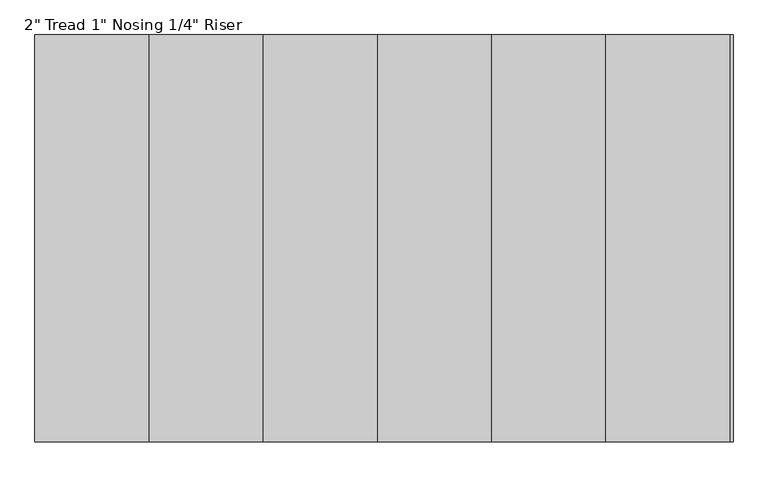
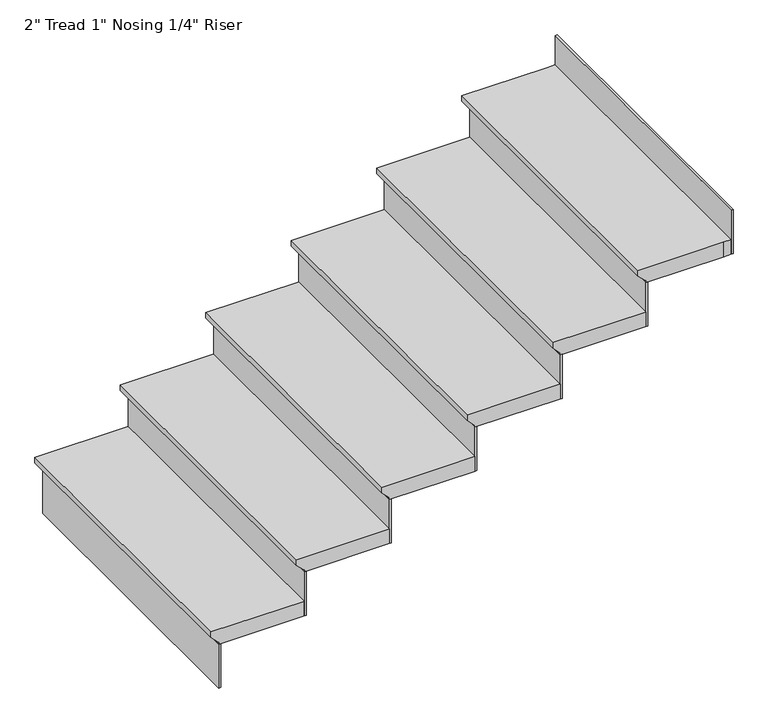
"""IFC4 building model written with IfcOpenShell, lengths in millimetres: stair flight geometry."""

from ifc_helpers import new_model, si_unit, origin, place, context, project, spatial, faceted_brep, source, transform, mapped, element, save


def stair_flight_d80cec9a(model_context):
    return source(origin(), model_context, "Body", "Brep", [
        faceted_brep([(-6729.7502524, 11195.5128362, 1352.55), (-6729.7502524, 11195.5128362, 1371.6), (-6729.7502524, 12192.4628362, 1371.6), (-6729.7502524, 12192.4628362, 1352.55), (-6704.3502524, 11195.5128362, 1327.15), (-6704.3502524, 12192.4628362, 1327.15), (-6424.9502524, 11195.5128362, 1371.6), (-6424.9502524, 12192.4628362, 1371.6), (-6704.3502524, 12192.4628362, 1320.8), (-6424.9502524, 12192.4628362, 1320.8), (-6424.9502524, 11195.5128362, 1320.8), (-6704.3502524, 11195.5128362, 1320.8)], [[[0, 1, 2, 3]], [[4, 0, 3, 5]], [[2, 1, 6, 7]], [[8, 9, 10, 11]], [[2, 7, 9, 8, 5, 3]], [[8, 11, 4, 5]], [[6, 1, 0, 4, 11, 10]], [[7, 6, 10, 9]]]),
        faceted_brep([(-6704.3502524, 11195.5128362, 1320.8), (-6704.3502524, 11195.5128362, 1168.4), (-6698.0002524, 11195.5128362, 1168.4), (-6698.0002524, 11195.5128362, 1320.8), (-6704.3502524, 12192.4628362, 1320.8), (-6698.0002524, 12192.4628362, 1320.8), (-6698.0002524, 12192.4628362, 1168.4), (-6704.3502524, 12192.4628362, 1168.4)], [[[0, 1, 2, 3]], [[4, 5, 6, 7]], [[1, 0, 4, 7]], [[2, 1, 7, 6]], [[3, 2, 6, 5]], [[0, 3, 5, 4]]]),
        faceted_brep([(-6424.9502524, 11195.5128362, 1473.2), (-6424.9502524, 11195.5128362, 1320.8), (-6418.6002524, 11195.5128362, 1320.8), (-6418.6002524, 11195.5128362, 1473.2), (-6424.9502524, 12192.4628362, 1473.2), (-6418.6002524, 12192.4628362, 1473.2), (-6418.6002524, 12192.4628362, 1320.8), (-6424.9502524, 12192.4628362, 1320.8)], [[[0, 1, 2, 3]], [[4, 5, 6, 7]], [[1, 0, 4, 7]], [[2, 1, 7, 6]], [[3, 2, 6, 5]], [[0, 3, 5, 4]]]),
        faceted_brep([(-6450.3502524, 12192.4628362, 1524.0), (-6450.3502524, 11195.5128362, 1524.0), (-6145.5502524, 11195.5128362, 1524.0), (-6145.5502524, 12192.4628362, 1524.0), (-6424.9502524, 12192.4628362, 1473.2), (-6145.5502524, 12192.4628362, 1473.2), (-6145.5502524, 11195.5128362, 1473.2), (-6424.9502524, 11195.5128362, 1473.2), (-6424.9502524, 12192.4628362, 1479.55), (-6450.3502524, 12192.4628362, 1504.95), (-6424.9502524, 11195.5128362, 1479.55), (-6450.3502524, 11195.5128362, 1504.95)], [[[0, 1, 2, 3]], [[4, 5, 6, 7]], [[0, 3, 5, 4, 8, 9]], [[4, 7, 10, 8]], [[2, 1, 11, 10, 7, 6]], [[3, 2, 6, 5]], [[11, 1, 0, 9]], [[10, 11, 9, 8]]]),
        faceted_brep([(-6145.5502524, 11195.5128362, 1625.6), (-6145.5502524, 11195.5128362, 1473.2), (-6139.2002524, 11195.5128362, 1473.2), (-6139.2002524, 11195.5128362, 1625.6), (-6145.5502524, 12192.4628362, 1625.6), (-6139.2002524, 12192.4628362, 1625.6), (-6139.2002524, 12192.4628362, 1473.2), (-6145.5502524, 12192.4628362, 1473.2)], [[[0, 1, 2, 3]], [[4, 5, 6, 7]], [[1, 0, 4, 7]], [[2, 1, 7, 6]], [[3, 2, 6, 5]], [[0, 3, 5, 4]]]),
        faceted_brep([(-6170.9502524, 12192.4628362, 1676.4), (-6170.9502524, 11195.5128362, 1676.4), (-5866.1502524, 11195.5128362, 1676.4), (-5866.1502524, 12192.4628362, 1676.4), (-6145.5502524, 12192.4628362, 1625.6), (-5866.1502524, 12192.4628362, 1625.6), (-5866.1502524, 11195.5128362, 1625.6), (-6145.5502524, 11195.5128362, 1625.6), (-6145.5502524, 12192.4628362, 1631.95), (-6170.9502524, 12192.4628362, 1657.35), (-6145.5502524, 11195.5128362, 1631.95), (-6170.9502524, 11195.5128362, 1657.35)], [[[0, 1, 2, 3]], [[4, 5, 6, 7]], [[0, 3, 5, 4, 8, 9]], [[4, 7, 10, 8]], [[2, 1, 11, 10, 7, 6]], [[3, 2, 6, 5]], [[11, 1, 0, 9]], [[10, 11, 9, 8]]]),
        faceted_brep([(-5866.1502524, 11195.5128362, 1778.0), (-5866.1502524, 11195.5128362, 1625.6), (-5859.8002524, 11195.5128362, 1625.6), (-5859.8002524, 11195.5128362, 1778.0), (-5866.1502524, 12192.4628362, 1778.0), (-5859.8002524, 12192.4628362, 1778.0), (-5859.8002524, 12192.4628362, 1625.6), (-5866.1502524, 12192.4628362, 1625.6)], [[[0, 1, 2, 3]], [[4, 5, 6, 7]], [[1, 0, 4, 7]], [[2, 1, 7, 6]], [[3, 2, 6, 5]], [[0, 3, 5, 4]]]),
        faceted_brep([(-5891.5502524, 12192.4628362, 1828.8), (-5891.5502524, 11195.5128362, 1828.8), (-5586.7502524, 11195.5128362, 1828.8), (-5586.7502524, 12192.4628362, 1828.8), (-5866.1502524, 12192.4628362, 1778.0), (-5586.7502524, 12192.4628362, 1778.0), (-5586.7502524, 11195.5128362, 1778.0), (-5866.1502524, 11195.5128362, 1778.0), (-5866.1502524, 12192.4628362, 1784.35), (-5891.5502524, 12192.4628362, 1809.75), (-5866.1502524, 11195.5128362, 1784.35), (-5891.5502524, 11195.5128362, 1809.75)], [[[0, 1, 2, 3]], [[4, 5, 6, 7]], [[0, 3, 5, 4, 8, 9]], [[4, 7, 10, 8]], [[2, 1, 11, 10, 7, 6]], [[3, 2, 6, 5]], [[11, 1, 0, 9]], [[10, 11, 9, 8]]]),
        faceted_brep([(-5586.7502524, 11195.5128362, 1930.4), (-5586.7502524, 11195.5128362, 1778.0), (-5580.4002524, 11195.5128362, 1778.0), (-5580.4002524, 11195.5128362, 1930.4), (-5586.7502524, 12192.4628362, 1930.4), (-5580.4002524, 12192.4628362, 1930.4), (-5580.4002524, 12192.4628362, 1778.0), (-5586.7502524, 12192.4628362, 1778.0)], [[[0, 1, 2, 3]], [[4, 5, 6, 7]], [[1, 0, 4, 7]], [[2, 1, 7, 6]], [[3, 2, 6, 5]], [[0, 3, 5, 4]]]),
        faceted_brep([(-5612.1502524, 12192.4628362, 1981.2), (-5612.1502524, 11195.5128362, 1981.2), (-5307.3502524, 11195.5128362, 1981.2), (-5307.3502524, 12192.4628362, 1981.2), (-5586.7502524, 12192.4628362, 1930.4), (-5307.3502524, 12192.4628362, 1930.4), (-5307.3502524, 11195.5128362, 1930.4), (-5586.7502524, 11195.5128362, 1930.4), (-5586.7502524, 12192.4628362, 1936.75), (-5612.1502524, 12192.4628362, 1962.15), (-5586.7502524, 11195.5128362, 1936.75), (-5612.1502524, 11195.5128362, 1962.15)], [[[0, 1, 2, 3]], [[4, 5, 6, 7]], [[0, 3, 5, 4, 8, 9]], [[4, 7, 10, 8]], [[2, 1, 11, 10, 7, 6]], [[3, 2, 6, 5]], [[11, 1, 0, 9]], [[10, 11, 9, 8]]]),
        faceted_brep([(-5027.9502524, 11195.5128362, 2235.2), (-5027.9502524, 11195.5128362, 2082.8), (-5021.6002524, 11195.5128362, 2082.8), (-5021.6002524, 11195.5128362, 2235.2), (-5027.9502524, 12192.4628362, 2235.2), (-5021.6002524, 12192.4628362, 2235.2), (-5021.6002524, 12192.4628362, 2082.8), (-5027.9502524, 12192.4628362, 2082.8)], [[[0, 1, 2, 3]], [[4, 5, 6, 7]], [[1, 0, 4, 7]], [[2, 1, 7, 6]], [[3, 2, 6, 5]], [[0, 3, 5, 4]]]),
        faceted_brep([(-5307.3502524, 11195.5128362, 2082.8), (-5307.3502524, 11195.5128362, 1930.4), (-5301.0002524, 11195.5128362, 1930.4), (-5301.0002524, 11195.5128362, 2082.8), (-5307.3502524, 12192.4628362, 2082.8), (-5301.0002524, 12192.4628362, 2082.8), (-5301.0002524, 12192.4628362, 1930.4), (-5307.3502524, 12192.4628362, 1930.4)], [[[0, 1, 2, 3]], [[4, 5, 6, 7]], [[1, 0, 4, 7]], [[2, 1, 7, 6]], [[3, 2, 6, 5]], [[0, 3, 5, 4]]]),
        faceted_brep([(-5027.9502524, 12192.4628362, 2133.6), (-5053.3502524, 12192.4628362, 2133.6), (-5332.7502524, 12192.4628362, 2133.6), (-5332.7502524, 11195.5128362, 2133.6), (-5053.3502524, 11195.5128362, 2133.6), (-5027.9502524, 11195.5128362, 2133.6), (-5053.3502524, 12192.4628362, 2082.8), (-5027.9502524, 12192.4628362, 2082.8), (-5027.9502524, 11195.5128362, 2082.8), (-5053.3502524, 11195.5128362, 2082.8), (-5307.3502524, 11195.5128362, 2082.8), (-5307.3502524, 12192.4628362, 2082.8), (-5307.3502524, 12192.4628362, 2089.15), (-5332.7502524, 12192.4628362, 2114.55), (-5307.3502524, 11195.5128362, 2089.15), (-5332.7502524, 11195.5128362, 2114.55)], [[[0, 1, 2, 3, 4, 5]], [[6, 7, 8, 9, 10, 11]], [[1, 0, 7, 6]], [[2, 1, 6, 11, 12, 13]], [[11, 10, 14, 12]], [[4, 3, 15, 14, 10, 9]], [[5, 4, 9, 8]], [[0, 5, 8, 7]], [[15, 3, 2, 13]], [[14, 15, 13, 12]]]),
    ])


if __name__ == "__main__":
    model = new_model("IFC4")
    model_context = context("Model", 3, world=origin())
    ifc_project = project(units=[si_unit("LENGTHUNIT", "METRE", prefix="MILLI")], contexts=[model_context])
    site = spatial("IfcSite", under=ifc_project)
    building = spatial("IfcBuilding", under=site)
    placement = place(None, origin())
    stair_flight_shape = stair_flight_d80cec9a(model_context)
    element("IfcStairFlight", 1, ObjectType="2\" Tread 1\" Nosing 1/4\" Riser", at=placement, inside=building, context=model_context, shape_type="MappedRepresentation", body=[
        mapped(stair_flight_shape, transform((0.0, 0.0, 0.0), x_axis=(1.0, 0.0, 0.0), y_axis=(0.0, 1.0, 0.0), z_axis=(0.0, 0.0, 1.0))),
    ])
    save(model, "model.ifc")
